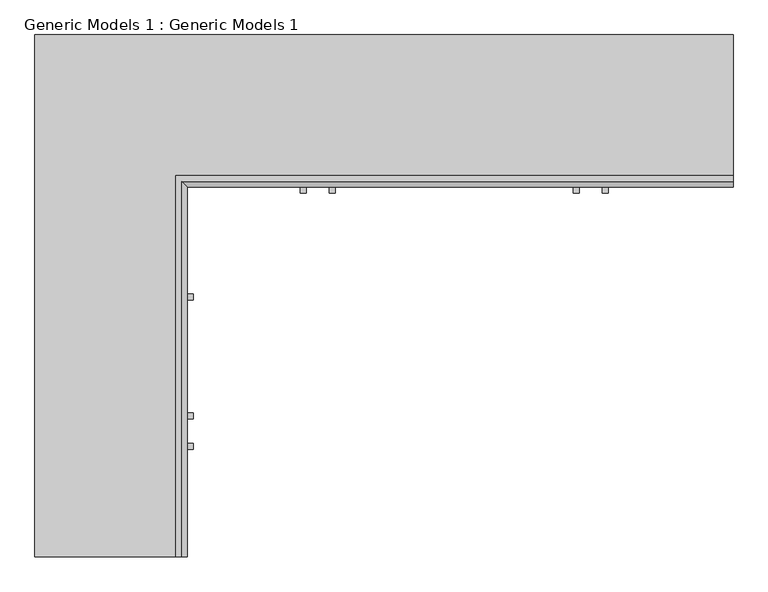
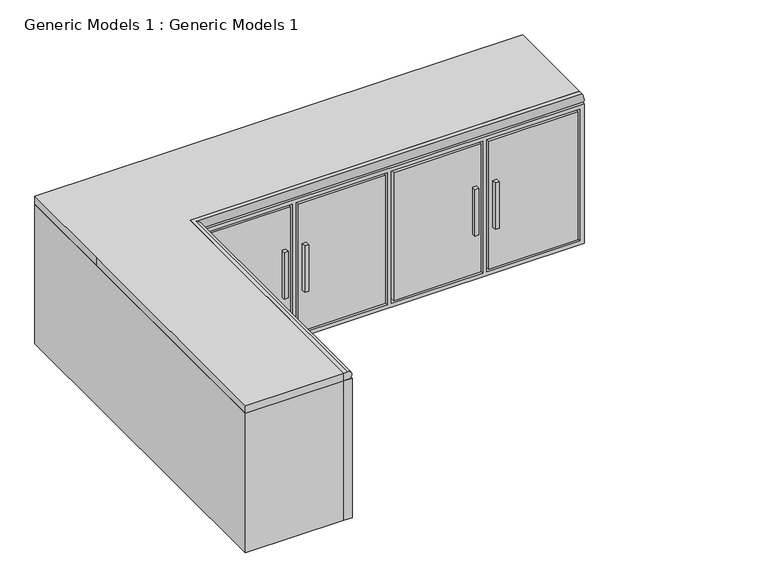
"""IFC4 building model written with IfcOpenShell, lengths in millimetres: proxy geometry, Generic Models 1 : Generic Models 1."""

from ifc_helpers import new_model, si_unit, frame, origin, origin_with_axes, place, context, project, spatial, polyline, circle_curve, ellipse_curve, outline, extrude, source, transform, mapped, element, save
from ifc_brep_helpers import plane_surface, cylinder_surface, advanced_brep


def generic_models_1_generic_models_1_c6f2978c(model_context):
    return source(origin(), model_context, "Body", "SolidModel", [
        extrude(outline(polyline([(-6654.2201068, 4079.2543681), (-6654.2201068, 4053.8543681), (-6679.6201068, 4053.8543681), (-6679.6201068, 4079.2543681), (-6654.2201068, 4079.2543681)])), frame((0.0, 0.0, 294.0134083), z_axis=(0.0, 0.0, 1.0), x_axis=(1.0, 0.0, 0.0)), (0.0, 0.0, 1.0), 304.8),
        extrude(outline(polyline([(-6654.2201068, 4210.0818146), (-6654.2201068, 4184.6818146), (-6679.6201068, 4184.6818146), (-6679.6201068, 4210.0818146), (-6654.2201068, 4210.0818146)])), frame((0.0, 0.0, 294.0134083), z_axis=(0.0, 0.0, 1.0), x_axis=(1.0, 0.0, 0.0)), (0.0, 0.0, 1.0), 304.8),
        extrude(outline(polyline([(-6654.2201068, 4726.5484812), (-6654.2201068, 4701.1484812), (-6679.6201068, 4701.1484812), (-6679.6201068, 4726.5484812), (-6654.2201068, 4726.5484812)])), frame((0.0, 0.0, 294.0134083), z_axis=(0.0, 0.0, 1.0), x_axis=(1.0, 0.0, 0.0)), (0.0, 0.0, 1.0), 304.8),
        extrude(outline(polyline([(-6679.6201068, 4104.6543681), (-6679.6201068, 3626.2877014), (-6730.4201068, 3626.2877014), (-6730.4201068, 4104.6543681), (-6679.6201068, 4104.6543681)])), frame((0.0, 0.0, 38.1), z_axis=(0.0, 0.0, 1.0), x_axis=(1.0, 0.0, 0.0)), (0.0, 0.0, 1.0), 838.2),
        extrude(outline(polyline([(-6679.6201068, 4621.1210347), (-6679.6201068, 4155.4543681), (-6730.4201068, 4155.4543681), (-6730.4201068, 4621.1210347), (-6679.6201068, 4621.1210347)])), frame((0.0, 0.0, 38.1), z_axis=(0.0, 0.0, 1.0), x_axis=(1.0, 0.0, 0.0)), (0.0, 0.0, 1.0), 838.2),
        extrude(outline(polyline([(-6679.6201068, 5150.2877014), (-6679.6201068, 4671.9210347), (-6730.4201068, 4671.9210347), (-6730.4201068, 5150.2877014), (-6679.6201068, 5150.2877014)])), frame((0.0, 0.0, 38.1), z_axis=(0.0, 0.0, 1.0), x_axis=(1.0, 0.0, 0.0)), (0.0, 0.0, 1.0), 838.2),
        extrude(outline(polyline([(-6165.2701068, 5162.9877014), (-6190.6701068, 5162.9877014), (-6190.6701068, 5188.3877014), (-6165.2701068, 5188.3877014), (-6165.2701068, 5162.9877014)])), frame((0.0, 0.0, 304.8), z_axis=(0.0, 0.0, 1.0), x_axis=(1.0, 0.0, 0.0)), (0.0, 0.0, 1.0), 304.8),
        extrude(outline(polyline([(-6039.4461066, 5162.9877014), (-6064.8461066, 5162.9877014), (-6064.8461066, 5188.3877014), (-6039.4461066, 5188.3877014), (-6039.4461066, 5162.9877014)])), frame((0.0, 0.0, 304.8), z_axis=(0.0, 0.0, 1.0), x_axis=(1.0, 0.0, 0.0)), (0.0, 0.0, 1.0), 304.8),
        extrude(outline(polyline([(-4984.1701068, 5162.9877014), (-5009.5701068, 5162.9877014), (-5009.5701068, 5188.3877014), (-4984.1701068, 5188.3877014), (-4984.1701068, 5162.9877014)])), frame((0.0, 0.0, 304.8), z_axis=(0.0, 0.0, 1.0), x_axis=(1.0, 0.0, 0.0)), (0.0, 0.0, 1.0), 304.8),
        extrude(outline(polyline([(-4858.3461066, 5162.9877014), (-4883.7461066, 5162.9877014), (-4883.7461066, 5188.3877014), (-4858.3461066, 5188.3877014), (-4858.3461066, 5162.9877014)])), frame((0.0, 0.0, 304.8), z_axis=(0.0, 0.0, 1.0), x_axis=(1.0, 0.0, 0.0)), (0.0, 0.0, 1.0), 304.8),
        extrude(outline(polyline([(-4355.5201068, 5188.3877014), (-4907.9701068, 5188.3877014), (-4907.9701068, 5239.1877014), (-4355.5201068, 5239.1877014), (-4355.5201068, 5188.3877014)])), frame((0.0, 0.0, 38.1), z_axis=(0.0, 0.0, 1.0), x_axis=(1.0, 0.0, 0.0)), (0.0, 0.0, 1.0), 838.2),
        extrude(outline(polyline([(-4958.7701068, 5188.3877014), (-5498.5201068, 5188.3877014), (-5498.5201068, 5239.1877014), (-4958.7701068, 5239.1877014), (-4958.7701068, 5188.3877014)])), frame((0.0, 0.0, 38.1), z_axis=(0.0, 0.0, 1.0), x_axis=(1.0, 0.0, 0.0)), (0.0, 0.0, 1.0), 838.2),
        extrude(outline(polyline([(-5549.3201068, 5188.3877014), (-6089.0701068, 5188.3877014), (-6089.0701068, 5239.1877014), (-5549.3201068, 5239.1877014), (-5549.3201068, 5188.3877014)])), frame((0.0, 0.0, 38.1), z_axis=(0.0, 0.0, 1.0), x_axis=(1.0, 0.0, 0.0)), (0.0, 0.0, 1.0), 838.2),
        extrude(outline(polyline([(-6139.8701068, 5188.3877014), (-6692.3201068, 5188.3877014), (-6692.3201068, 5239.1877014), (-6139.8701068, 5239.1877014), (-6139.8701068, 5188.3877014)])), frame((0.0, 0.0, 38.1), z_axis=(0.0, 0.0, 1.0), x_axis=(1.0, 0.0, 0.0)), (0.0, 0.0, 1.0), 838.2),
        extrude(outline(polyline([(5188.3877014, 914.4), (5188.3877014, 0.0), (3588.1877014, 0.0), (3588.1877014, 914.4), (5188.3877014, 914.4)]), holes=[polyline([(4659.2210347, 25.4), (5162.9877014, 25.4), (5162.9877014, 889.0), (4659.2210347, 889.0), (4659.2210347, 25.4)]), polyline([(4117.3543681, 889.0), (3613.5877014, 889.0), (3613.5877014, 25.4), (4117.3543681, 25.4), (4117.3543681, 889.0)]), polyline([(4142.7543681, 25.4), (4633.8210347, 25.4), (4633.8210347, 889.0), (4142.7543681, 889.0), (4142.7543681, 25.4)])]), frame((-6730.4201068, 0.0, 0.0), z_axis=(1.0, 0.0, 0.0), x_axis=(0.0, 1.0, 0.0)), (0.0, 0.0, 1.0), 50.8),
        extrude(outline(polyline([(0.0, -6730.4201068), (0.0, -4317.4201068), (914.4, -4317.4201068), (914.4, -6730.4201068), (0.0, -6730.4201068)]), holes=[polyline([(889.0, -6127.1701068), (25.4, -6127.1701068), (25.4, -6705.0201068), (889.0, -6705.0201068), (889.0, -6127.1701068)]), polyline([(25.4, -4920.6701068), (889.0, -4920.6701068), (889.0, -4342.8201068), (25.4, -4342.8201068), (25.4, -4920.6701068)]), polyline([(25.4, -6101.7701068), (889.0, -6101.7701068), (889.0, -5536.6201068), (25.4, -5536.6201068), (25.4, -6101.7701068)]), polyline([(25.4, -5511.2201068), (889.0, -5511.2201068), (889.0, -4946.0701068), (25.4, -4946.0701068), (25.4, -5511.2201068)])]), frame((0.0, 5188.3877014, 0.0), z_axis=(0.0, 1.0, 0.0), x_axis=(0.0, 0.0, 1.0)), (0.0, 0.0, 1.0), 50.8),
        advanced_brep(
        [(-6730.4201068, 3588.1877014, 914.4), (-6705.0201068, 3588.1877014, 914.4), (-6705.0201068, 3588.1877014, 965.2), (-6730.4201068, 3588.1877014, 965.2), (-6730.4201068, 5239.1877014, 914.4), (-4317.4201068, 5239.1877014, 914.4), (-4317.4201068, 5213.7877014, 914.4), (-6705.0201068, 5213.7877014, 914.4), (-6705.0201068, 5213.7877014, 965.2), (-4317.4201068, 5213.7877014, 965.2), (-4317.4201068, 5239.1877014, 965.2), (-6730.4201068, 5239.1877014, 965.2)],
        [
            (0, 1),
            (1, 2, circle_curve(frame((-6705.0201068, 3588.1877014, 939.8), z_axis=(0.0, -1.0, 0.0), x_axis=(-1.0, 0.0, 0.0)), 25.4)),
            (2, 3),
            (3, 0),
            (0, 4),
            (4, 5),
            (5, 6),
            (6, 7),
            (7, 1),
            (7, 8, ellipse_curve(frame((-6705.0201068, 5213.7877014, 939.8), z_axis=(-0.707106781186549, -0.7071067811865459, 0.0), x_axis=(0.7071067811865458, -0.7071067811865492, 0.0)), 35.9210245, 25.4)),
            (8, 2),
            (8, 9),
            (9, 10),
            (10, 11),
            (11, 3),
            (11, 4),
            (5, 10),
            (9, 6, circle_curve(frame((-4317.4201068, 5213.7877014, 939.8), z_axis=(1.0, 0.0, 0.0), x_axis=(0.0, 1.0, 0.0)), 25.4)),
        ],
        [
            plane_surface(frame((-6730.4201068, 3588.1877014, -609.6), z_axis=(0.0, -1.0, 0.0), x_axis=(0.0, 0.0, 1.0))),
            plane_surface(frame((-6730.4201068, 3588.1877014, 914.4), z_axis=(0.0, 0.0, -1.0), x_axis=(0.0, 1.0, 0.0))),
            cylinder_surface(frame((-6705.0201068, 3588.1877014, 939.8), z_axis=(0.0, -1.0, 0.0), x_axis=(-1.0, 0.0, 0.0)), 25.4),
            plane_surface(frame((-6705.0201068, 3588.1877014, 965.2), z_axis=(0.0, 0.0, 1.0), x_axis=(0.0, 1.0, 0.0))),
            plane_surface(frame((-6730.4201068, 3588.1877014, 965.2), z_axis=(-1.0, 0.0, 0.0), x_axis=(0.0, 1.0, 0.0))),
            plane_surface(frame((-4317.4201068, 5239.1877014, -609.6), z_axis=(1.0, 0.0, 0.0), x_axis=(0.0, 0.0, 1.0))),
            cylinder_surface(frame((-6730.4201068, 5213.7877014, 939.8), z_axis=(-1.0, 0.0, 0.0), x_axis=(0.0, 1.0, 0.0)), 25.4),
            plane_surface(frame((-6730.4201068, 5239.1877014, 965.2), z_axis=(0.0, 1.0, 0.0), x_axis=(1.0, 0.0, 0.0))),
        ],
        [
            (0, [[1, 2, 3, 4]]),
            (1, [[-1, 5, 6, 7, 8, 9]]),
            (2, [[-2, -9, 10, 11]]),
            (3, [[-3, -11, 12, 13, 14, 15]]),
            (4, [[-4, -15, 16, -5]]),
            (5, [[17, -13, 18, -7]]),
            (6, [[-10, -8, -18, -12]]),
            (7, [[-16, -14, -17, -6]]),
        ],
    ),
        extrude(outline(polyline([(-6730.4201068, 5239.1877014), (-6730.4201068, 3588.1877014), (-7340.0201068, 3588.1877014), (-7340.0201068, 5188.3877014), (-7340.0201068, 5848.7877014), (-4317.4201068, 5848.7877014), (-4317.4201068, 5239.1877014), (-6730.4201068, 5239.1877014)])), frame((0.0, 0.0, 914.4), z_axis=(0.0, 0.0, 1.0), x_axis=(1.0, 0.0, 0.0)), (0.0, 0.0, 1.0), 50.8),
        extrude(outline(polyline([(-6730.4201068, 3588.1877014), (-7340.0201068, 3588.1877014), (-7340.0201068, 5848.7877014), (-6730.4201068, 5848.7877014), (-4317.4201068, 5848.7877014), (-4317.4201068, 5239.1877014), (-6730.4201068, 5239.1877014), (-6730.4201068, 3588.1877014)])), origin_with_axes(), (0.0, 0.0, 1.0), 914.4),
    ])


if __name__ == "__main__":
    model = new_model("IFC4")
    model_context = context("Model", 3, world=origin())
    ifc_project = project(units=[si_unit("LENGTHUNIT", "METRE", prefix="MILLI")], contexts=[model_context])
    site = spatial("IfcSite", under=ifc_project)
    building = spatial("IfcBuilding", under=site)
    placement = place(None, origin())
    generic_models_1_generic_models_1_shape = generic_models_1_generic_models_1_c6f2978c(model_context)
    element("IfcBuildingElementProxy", 1, Name="Generic Models 1 : Generic Models 1", ObjectType="Generic Models 1 : Generic Models 1", at=placement, inside=building, context=model_context, shape_type="MappedRepresentation", body=[
        mapped(generic_models_1_generic_models_1_shape, transform((0.0, 0.0, 0.0), x_axis=(1.0, 0.0, 0.0), y_axis=(0.0, 1.0, 0.0), z_axis=(0.0, 0.0, 1.0))),
    ])
    save(model, "model.ifc")

# Revit data of these elements
# Element 1 (IfcBuildingElementProxy, "Generic Models 1 : Generic Models 1")
#   Materials on its faces: "0 kitchen tiles(1)", "0 kitchen tiles(2)", "0 kitchen tiles(3)", "0 kitchen tiles"
# Materials
#   "0 kitchen tiles(1)": class "Generic", colour RGB 120 120 120, transparency 0, Cost = 0
#   "0 kitchen tiles(2)": class "Generic", colour RGB 120 120 120, transparency 0, Cost = 0
#   "0 kitchen tiles(3)": class "Generic", colour RGB 120 120 120, transparency 0, Cost = 0
#   "0 kitchen tiles": class "Generic", colour RGB 120 120 120, transparency 0, Cost = 0
